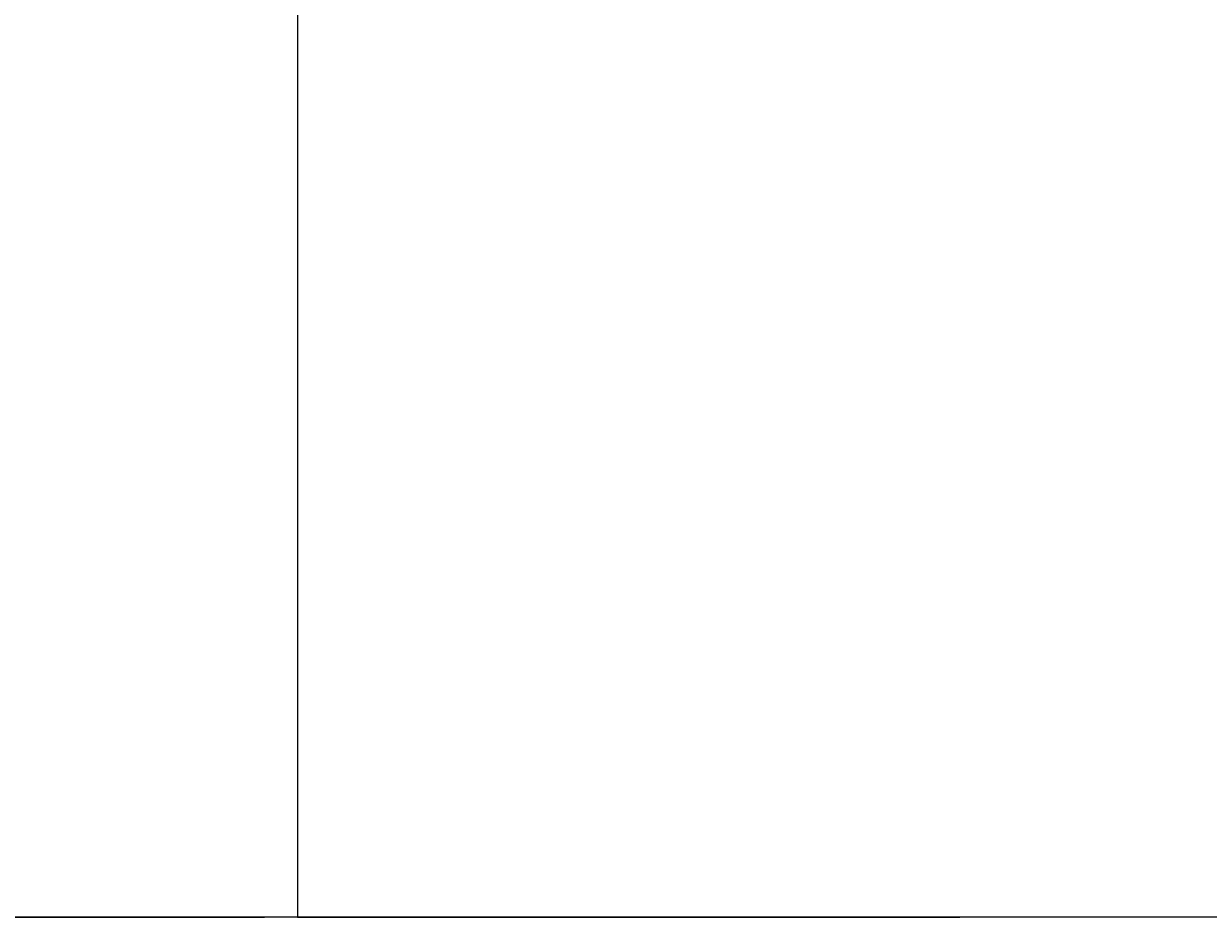
# Model space of a CAD drawing. Units: inches. Extents: x 35362 to 73946, y 43607 to 67532.
# Tile 133 of 134: x 64925 to 66704, y 43607 to 44948. Entities that reach past the tile are written whole.
import ezdxf

# ---------------------------------------------------------------- set-up
doc = ezdxf.new("R2010")
doc.units = ezdxf.units.IN
doc.header["$MEASUREMENT"] = 0
doc.layers.add('A-ANNO-DIMS', color=2, linetype='Continuous', lineweight=18)
doc.styles.get("Standard").update_dxf_attribs({"font": 'arial.ttf'})
doc.dimstyles.get("Standard").update_dxf_attribs({"dimtxt": 0.18, "dimasz": 0.18, "dimexe": 0.18, "dimexo": 0.0625, "dimgap": 0.09, "dimtad": 0, "dimtih": 1, "dimtoh": 1, "dimdec": 4, "dimzin": 0, "dimdsep": 46, "dimtxsty": 'Standard', "dimcen": 0.09, "dimadec": 0, "dimazin": 0, "dimtfac": 1, "dimtdec": 4, "dimtofl": 0, "dimtmove": 0, "dimatfit": 3, "dimfxl": 1, "dimtolj": 1, "dimtzin": 0, "dimarcsym": 0})

# ---------------------------------------------------------------- blocks, each defined once
blk = doc.blocks.new('*D5')
at = {"layer": 'A-ANNO-DIMS', "color": 0, "lineweight": -2, "transparency": 16777216}
for p, q in [((37121.949085, 46919.318283), (37121.949085, 43606.678996)), ((69871.496302, 45449.831951), (69871.496302, 43606.678996)), ((37122.129085, 43606.858996), (53496.2943647142, 43606.858996)), ((69871.316302, 43606.858996), (53497.15102228581, 43606.858996))]:
    blk.add_line(p, q, dxfattribs=at)
at = {"layer": 'A-ANNO-DIMS', "color": 0, "transparency": 16777216}
for points in [[(37122.129085, 43606.888996), (37122.129085, 43606.828996), (37121.949085, 43606.858996)], [(69871.316302, 43606.888996), (69871.316302, 43606.828996), (69871.496302, 43606.858996)]]:
    blk.add_solid(points, dxfattribs=at)
at = {"layer": 'Defpoints', "color": 0, "transparency": 16777216}
for p in [(37121.949085, 46919.380783), (69871.496302, 45449.894451), (69871.496302, 43606.858996)]:
    blk.add_point(p, dxfattribs=at)
at = {"layer": 'A-ANNO-DIMS', "color": 0, "transparency": 16777216, "insert": (53496.7226935, 43606.858996), "char_height": 0.18, "attachment_point": 5}
blk.add_mtext('\\A1;32750', dxfattribs=at)
blk = doc.blocks.new('*D38')
at = {"layer": 'A-ANNO-DIMS', "color": 0, "lineweight": -2, "transparency": 16777216}
for p, q in [((68483.500128, 45449.831951), (68483.500128, 43606.678996)), ((62090.58505699999, 45366.796496), (62090.58505699999, 43606.678996)), ((62090.76505699999, 43606.858996), (65286.57828827081, 43606.858996)), ((68483.320128, 43606.858996), (65287.5068967292, 43606.858996))]:
    blk.add_line(p, q, dxfattribs=at)
at = {"layer": 'A-ANNO-DIMS', "color": 0, "transparency": 16777216}
for points in [[(62090.76505699999, 43606.888996), (62090.76505699999, 43606.828996), (62090.58505699999, 43606.858996)], [(68483.320128, 43606.888996), (68483.320128, 43606.828996), (68483.500128, 43606.858996)]]:
    blk.add_solid(points, dxfattribs=at)
at = {"layer": 'Defpoints', "color": 0, "transparency": 16777216}
for p in [(68483.500128, 45449.894451), (62090.58505699999, 45366.858996), (68483.500128, 43606.858996)]:
    blk.add_point(p, dxfattribs=at)
at = {"layer": 'A-ANNO-DIMS', "color": 0, "transparency": 16777216, "insert": (65287.0425925, 43606.858996), "char_height": 0.18, "attachment_point": 5}
blk.add_mtext('\\A1;6392.9', dxfattribs=at)
blk = doc.blocks.new('*D65')
at = {"layer": 'A-ANNO-DIMS', "color": 0, "lineweight": -2, "transparency": 16777216}
for p, q in [((65336.01600799999, 61293.223552), (65336.01600799999, 43606.678996)), ((67326.639741, 61293.223552), (67326.639741, 43606.678996)), ((65336.19600799999, 43606.858996), (66330.87277900206, 43606.858996)), ((67326.45974100001, 43606.858996), (66331.78296999796, 43606.858996))]:
    blk.add_line(p, q, dxfattribs=at)
at = {"layer": 'A-ANNO-DIMS', "color": 0, "transparency": 16777216}
for points in [[(65336.19600799999, 43606.888996), (65336.19600799999, 43606.828996), (65336.01600799999, 43606.858996)], [(67326.45974100001, 43606.888996), (67326.45974100001, 43606.828996), (67326.639741, 43606.858996)]]:
    blk.add_solid(points, dxfattribs=at)
at = {"layer": 'Defpoints', "color": 0, "transparency": 16777216}
for p in [(65336.01600799999, 61293.286052), (67326.639741, 61293.286052), (67326.639741, 43606.858996)]:
    blk.add_point(p, dxfattribs=at)
at = {"layer": 'A-ANNO-DIMS', "color": 0, "transparency": 16777216, "insert": (66331.32787450001, 43606.858996), "char_height": 0.18, "attachment_point": 5}
blk.add_mtext('\\A1;1990.6', dxfattribs=at)
blk = doc.blocks.new('*D68')
at = {"layer": 'A-ANNO-DIMS', "color": 0, "lineweight": -2, "transparency": 16777216}
for p, q in [((68320.870762, 54372.885224), (68320.870762, 43606.678996)), ((61240.907336, 53351.466162), (61240.907336, 43606.678996)), ((61241.08733599999, 43606.858996), (64780.42646373397, 43606.858996)), ((68320.69076200001, 43606.858996), (64781.35163426603, 43606.858996))]:
    blk.add_line(p, q, dxfattribs=at)
at = {"layer": 'A-ANNO-DIMS', "color": 0, "transparency": 16777216}
for points in [[(61241.08733599999, 43606.888996), (61241.08733599999, 43606.828996), (61240.907336, 43606.858996)], [(68320.69076200001, 43606.888996), (68320.69076200001, 43606.828996), (68320.870762, 43606.858996)]]:
    blk.add_solid(points, dxfattribs=at)
at = {"layer": 'Defpoints', "color": 0, "transparency": 16777216}
for p in [(68320.870762, 54372.947724), (61240.907336, 53351.52866199999), (68320.870762, 43606.858996)]:
    blk.add_point(p, dxfattribs=at)
at = {"layer": 'A-ANNO-DIMS', "color": 0, "transparency": 16777216, "insert": (64780.889049, 43606.858996), "char_height": 0.18, "attachment_point": 5}
blk.add_mtext('\\A1;7080.0', dxfattribs=at)

msp = doc.modelspace()

# ---------------------------------------------------------------- dimensions: what is measured, and where the dimension line sits
at = {"layer": 'A-ANNO-DIMS'}
for base, p1, p2, override, picture, middle in [((67326.639741, 43606.858996), (65336.01600799999, 61293.286052), (67326.639741, 61293.286052), {"dimdec": 1, "dimlfac": 1, "dimrnd": 0, "dimzin": 0, "dimdsep": 46, "dimlunit": 2}, '*D65', (66331.32787450001, 43606.858996)), ((68320.870762, 43606.858996), (61240.907336, 53351.52866199999), (68320.870762, 54372.947724), {"dimdec": 1, "dimlfac": 1, "dimrnd": 0, "dimzin": 0, "dimdsep": 46, "dimlunit": 2}, '*D68', (64780.889049, 43606.858996)), ((69871.496302, 43606.858996), (37121.949085, 46919.380783), (69871.496302, 45449.894451), {"dimdec": 0, "dimlfac": 1, "dimrnd": 0, "dimzin": 0, "dimdsep": 46, "dimlunit": 2}, '*D5', (53496.7226935, 43606.858996)), ((68483.500128, 43606.858996), (62090.58505699999, 45366.858996), (68483.500128, 45449.894451), {"dimdec": 1, "dimlfac": 1, "dimrnd": 0, "dimzin": 0, "dimdsep": 46, "dimlunit": 2}, '*D38', (65287.0425925, 43606.858996))]:
    dim = msp.add_linear_dim(base=base, p1=p1, p2=p2, dimstyle='Standard', override=override, dxfattribs=at)
    dim.commit()
    dim.dimension.update_dxf_attribs({"geometry": picture, "text_midpoint": middle})

doc.saveas('drawing.dxf')
